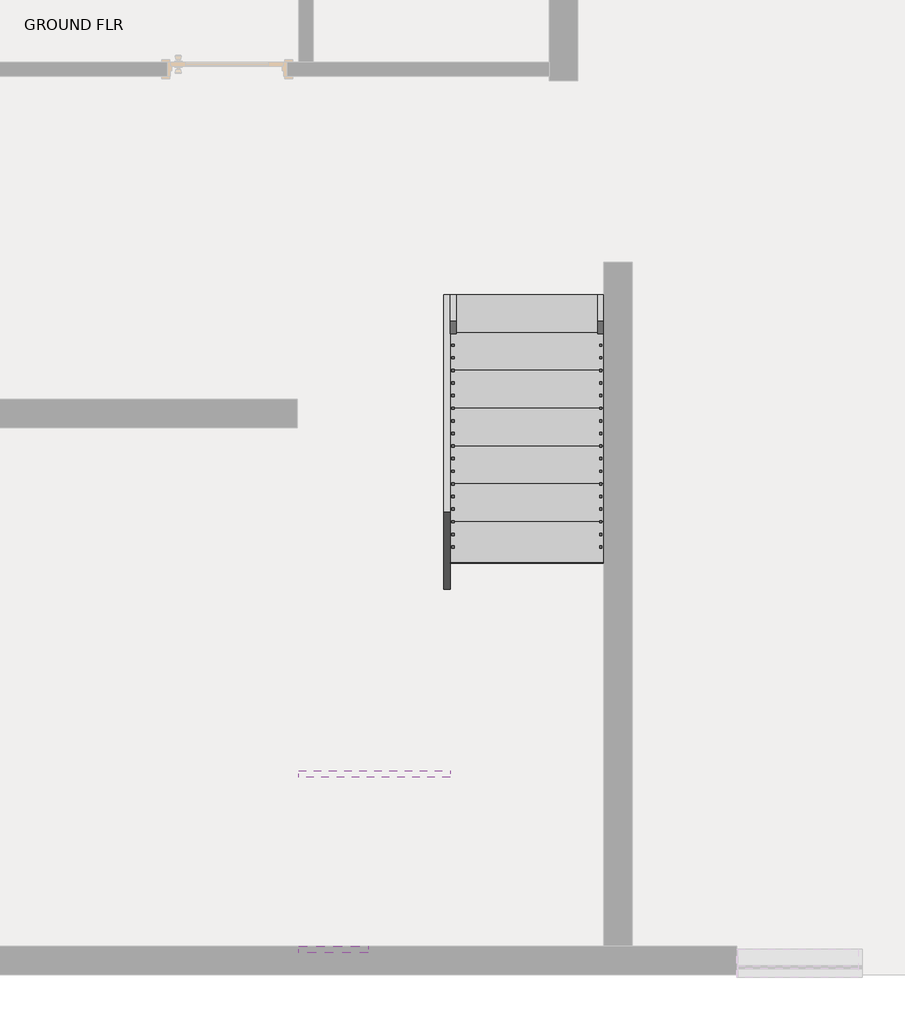
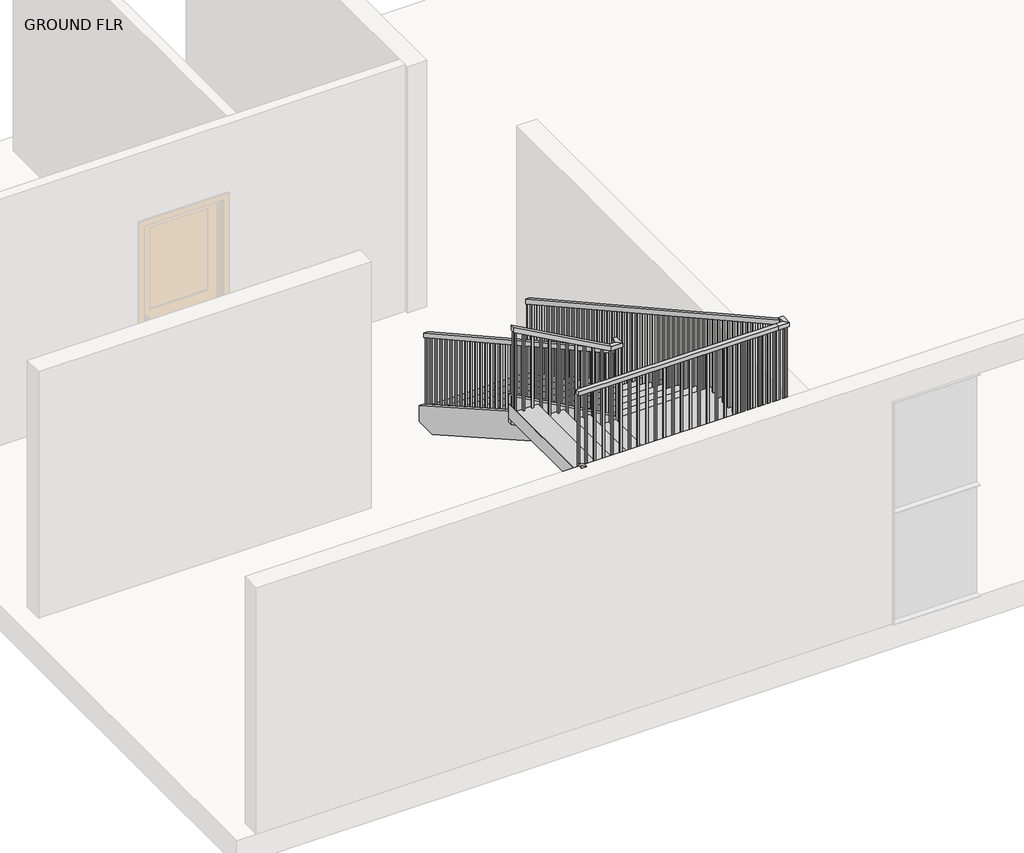
# One storey, part 3 of 3: 4 members, 2 railings, 1 stair flight.
"""IFC4 building model written with IfcOpenShell, lengths in millimetres."""

from ifc_helpers import new_model, si_unit, frame, origin, place, context, project, spatial, polyline, outline, extrude, faceted_brep, transform, mapped, element, save
from components import stair_flight_acf00c5d

model = new_model("IFC4")

# Units and contexts
model_context = context("Model", 3, world=origin())
ifc_project = project(units=[si_unit("LENGTHUNIT", "METRE", prefix="MILLI")], contexts=[model_context])

# Site, building, storey
site = spatial("IfcSite", under=ifc_project)
building = spatial("IfcBuilding", under=site)
storey = spatial("IfcBuildingStorey", under=building, Name="GROUND FLR", Elevation=304.8)

# Members
placement = place(None, origin())
element("IfcMember", 1, ObjectType="Stringer - 2\" Width", at=placement, inside=storey, context=model_context, shape_type="SweptSolid", body=[
    extrude(outline(polyline([(-746.7863315, 512.3983948), (-746.7863315, 304.8), (-1000.7308343, 304.8), (-4096.6287758, 2024.7433008), (-3469.0071624, 2024.7433008), (-746.7863315, 512.3983948)])), frame((-3766.7446058, 0.0, 0.0), z_axis=(1.0, 0.0, 0.0), x_axis=(0.0, 1.0, 0.0)), (0.0, 0.0, 1.0), 50.8),
])
element("IfcMember", 2, ObjectType="Stringer - 2\" Width", at=placement, inside=storey, context=model_context, shape_type="SweptSolid", body=[
    extrude(outline(polyline([(3080.0080444, -5666.2211442), (3391.0650614, -6226.1237749), (3080.0080444, -6226.1237749), (3080.0080444, -5666.2211442)])), frame((0.0, -6046.9053142, 0.0), z_axis=(0.0, 1.0, 0.0), x_axis=(0.0, 0.0, 1.0)), (0.0, 0.0, 1.0), 50.8),
])
element("IfcMember", 3, ObjectType="Stringer - 2\" Width", at=placement, inside=storey, context=model_context, shape_type="SweptSolid", body=[
    extrude(outline(polyline([(-746.7863315, 509.8166394), (-746.7863315, 304.8), (-1003.0994439, 304.8), (-4582.1863315, 2335.4875958), (-4582.1863315, 2685.9301146), (-746.7863315, 509.8166394)])), frame((-5057.7237749, 0.0, 0.0), z_axis=(1.0, 0.0, 0.0), x_axis=(0.0, 1.0, 0.0)), (0.0, 0.0, 1.0), 50.8),
])
element("IfcMember", 4, ObjectType="Stringer - 2\" Width", at=placement, inside=storey, context=model_context, shape_type="SweptSolid", body=[
    extrude(outline(polyline([(2365.053054, -5006.9237749), (2713.7317281, -5006.9237749), (3391.0650614, -6226.1237749), (3042.3863873, -6226.1237749), (2365.053054, -5006.9237749)])), frame((0.0, -4632.9863315, 0.0), z_axis=(0.0, 1.0, 0.0), x_axis=(0.0, 0.0, 1.0)), (0.0, 0.0, 1.0), 50.8),
])

# Railings
element("IfcRailing", 5, ObjectType="Handrail - Rectangular", at=placement, inside=storey, context=model_context, shape_type="SolidModel", body=[
    faceted_brep([(-4956.1237749, -746.7863315, 1388.5333333), (-4956.1237749, -746.7863315, 1330.420221), (-5006.9237749, -746.7863315, 1330.420221), (-5006.9237749, -746.7863315, 1388.5333333), (-4956.1237749, -4556.7863315, 3505.2), (-4956.1237749, -4607.5863315, 3475.3091099), (-5006.9237749, -4607.5863315, 3475.3091099), (-5006.9237749, -4556.7863315, 3505.2), (-4956.1237749, -4556.7863315, 3632.2), (-4956.1237749, -4607.5863315, 3581.4), (-5006.9237749, -4607.5863315, 3581.4), (-5006.9237749, -4556.7863315, 3632.2), (-4956.1237749, -4683.7863315, 3632.2), (-4956.1237749, -4683.7863315, 3581.4), (-5006.9237749, -4632.9863315, 3581.4), (-5006.9237749, -4632.9863315, 3632.2), (-5083.1237749, -4683.7863315, 3632.2), (-5096.2873772, -4683.7863315, 3581.4), (-5096.2873772, -4632.9863315, 3581.4), (-5083.1237749, -4632.9863315, 3632.2), (-6226.1237749, -4683.7863315, 4267.2), (-6226.1237749, -4632.9863315, 4267.2), (-6226.1237749, -4632.9863315, 4209.0868876), (-6226.1237749, -4683.7863315, 4209.0868876)], [[[0, 1, 2, 3]], [[1, 0, 4, 5]], [[2, 1, 5, 6]], [[3, 2, 6, 7]], [[0, 3, 7, 4]], [[5, 4, 8, 9]], [[6, 5, 9, 10]], [[7, 6, 10, 11]], [[4, 7, 11, 8]], [[9, 8, 12, 13]], [[10, 9, 13, 14]], [[11, 10, 14, 15]], [[8, 11, 15, 12]], [[13, 12, 16, 17]], [[14, 13, 17, 18]], [[15, 14, 18, 19]], [[12, 15, 19, 16]], [[20, 21, 22, 23]], [[17, 16, 20, 23]], [[18, 17, 23, 22]], [[19, 18, 22, 21]], [[16, 19, 21, 20]]]),
    extrude(outline(polyline([(4189.6841099, -6191.1987749), (4200.2674432, -6210.2487749), (3183.4666667, -6210.2487749), (3183.4666667, -6191.1987749), (4189.6841099, -6191.1987749)])), frame((0.0, -4667.9113315, 0.0), z_axis=(0.0, 1.0, 0.0), x_axis=(0.0, 0.0, 1.0)), (0.0, 0.0, 1.0), 19.05),
    extrude(outline(polyline([(4133.2396654, -6089.5987749), (4143.8229988, -6108.6487749), (3183.4666667, -6108.6487749), (3183.4666667, -6089.5987749), (4133.2396654, -6089.5987749)])), frame((0.0, -4667.9113315, 0.0), z_axis=(0.0, 1.0, 0.0), x_axis=(0.0, 0.0, 1.0)), (0.0, 0.0, 1.0), 19.05),
    extrude(outline(polyline([(4076.795221, -5987.9987749), (4087.3785543, -6007.0487749), (3183.4666667, -6007.0487749), (3183.4666667, -5987.9987749), (4076.795221, -5987.9987749)])), frame((0.0, -4667.9113315, 0.0), z_axis=(0.0, 1.0, 0.0), x_axis=(0.0, 0.0, 1.0)), (0.0, 0.0, 1.0), 19.05),
    extrude(outline(polyline([(4020.3507765, -5886.3987749), (4030.9341099, -5905.4487749), (3014.1333333, -5905.4487749), (3014.1333333, -5886.3987749), (4020.3507765, -5886.3987749)])), frame((0.0, -4667.9113315, 0.0), z_axis=(0.0, 1.0, 0.0), x_axis=(0.0, 0.0, 1.0)), (0.0, 0.0, 1.0), 19.05),
    extrude(outline(polyline([(3963.9063321, -5784.7987749), (3974.4896654, -5803.8487749), (3014.1333333, -5803.8487749), (3014.1333333, -5784.7987749), (3963.9063321, -5784.7987749)])), frame((0.0, -4667.9113315, 0.0), z_axis=(0.0, 1.0, 0.0), x_axis=(0.0, 0.0, 1.0)), (0.0, 0.0, 1.0), 19.05),
    extrude(outline(polyline([(3907.4618876, -5683.1987749), (3918.045221, -5702.2487749), (3014.1333333, -5702.2487749), (3014.1333333, -5683.1987749), (3907.4618876, -5683.1987749)])), frame((0.0, -4667.9113315, 0.0), z_axis=(0.0, 1.0, 0.0), x_axis=(0.0, 0.0, 1.0)), (0.0, 0.0, 1.0), 19.05),
    extrude(outline(polyline([(3851.0174432, -5581.5987749), (3861.6007765, -5600.6487749), (2844.8, -5600.6487749), (2844.8, -5581.5987749), (3851.0174432, -5581.5987749)])), frame((0.0, -4667.9113315, 0.0), z_axis=(0.0, 1.0, 0.0), x_axis=(0.0, 0.0, 1.0)), (0.0, 0.0, 1.0), 19.05),
    extrude(outline(polyline([(3794.5729988, -5479.9987749), (3805.1563321, -5499.0487749), (2844.8, -5499.0487749), (2844.8, -5479.9987749), (3794.5729988, -5479.9987749)])), frame((0.0, -4667.9113315, 0.0), z_axis=(0.0, 1.0, 0.0), x_axis=(0.0, 0.0, 1.0)), (0.0, 0.0, 1.0), 19.05),
    extrude(outline(polyline([(3738.1285543, -5378.3987749), (3748.7118876, -5397.4487749), (2844.8, -5397.4487749), (2844.8, -5378.3987749), (3738.1285543, -5378.3987749)])), frame((0.0, -4667.9113315, 0.0), z_axis=(0.0, 1.0, 0.0), x_axis=(0.0, 0.0, 1.0)), (0.0, 0.0, 1.0), 19.05),
    extrude(outline(polyline([(3681.6841099, -5276.7987749), (3692.2674432, -5295.8487749), (2675.4666667, -5295.8487749), (2675.4666667, -5276.7987749), (3681.6841099, -5276.7987749)])), frame((0.0, -4667.9113315, 0.0), z_axis=(0.0, 1.0, 0.0), x_axis=(0.0, 0.0, 1.0)), (0.0, 0.0, 1.0), 19.05),
    extrude(outline(polyline([(3625.2396654, -5175.1987749), (3635.8229988, -5194.2487749), (2675.4666667, -5194.2487749), (2675.4666667, -5175.1987749), (3625.2396654, -5175.1987749)])), frame((0.0, -4667.9113315, 0.0), z_axis=(0.0, 1.0, 0.0), x_axis=(0.0, 0.0, 1.0)), (0.0, 0.0, 1.0), 19.05),
    extrude(outline(polyline([(3568.795221, -5073.5987749), (3579.3785543, -5092.6487749), (2675.4666667, -5092.6487749), (2675.4666667, -5073.5987749), (3568.795221, -5073.5987749)])), frame((0.0, -4667.9113315, 0.0), z_axis=(0.0, 1.0, 0.0), x_axis=(0.0, 0.0, 1.0)), (0.0, 0.0, 1.0), 19.05),
    extrude(outline(polyline([(-4991.0487749, -4598.0613315), (-4971.9987749, -4598.0613315), (-4971.9987749, -4617.1113315), (-4991.0487749, -4617.1113315), (-4991.0487749, -4598.0613315)])), frame((0.0, 0.0, 2506.1333333), z_axis=(0.0, 0.0, 1.0), x_axis=(1.0, 0.0, 0.0)), (0.0, 0.0, 1.0), 1075.2666667),
    extrude(outline(polyline([(-4515.5113315, 3424.1563321), (-4496.4613315, 3413.5729988), (-4496.4613315, 2506.1333333), (-4515.5113315, 2506.1333333), (-4515.5113315, 3424.1563321)])), frame((-4991.0487749, 0.0, 0.0), z_axis=(1.0, 0.0, 0.0), x_axis=(0.0, 1.0, 0.0)), (0.0, 0.0, 1.0), 19.05),
    extrude(outline(polyline([(-4413.9113315, 3367.7118876), (-4394.8613315, 3357.1285543), (-4394.8613315, 2506.1333333), (-4413.9113315, 2506.1333333), (-4413.9113315, 3367.7118876)])), frame((-4991.0487749, 0.0, 0.0), z_axis=(1.0, 0.0, 0.0), x_axis=(0.0, 1.0, 0.0)), (0.0, 0.0, 1.0), 19.05),
    extrude(outline(polyline([(-4312.3113315, 3311.2674432), (-4293.2613315, 3300.6841099), (-4293.2613315, 2336.8), (-4312.3113315, 2336.8), (-4312.3113315, 3311.2674432)])), frame((-4991.0487749, 0.0, 0.0), z_axis=(1.0, 0.0, 0.0), x_axis=(0.0, 1.0, 0.0)), (0.0, 0.0, 1.0), 19.05),
    extrude(outline(polyline([(-4210.7113315, 3254.8229988), (-4191.6613315, 3244.2396654), (-4191.6613315, 2336.8), (-4210.7113315, 2336.8), (-4210.7113315, 3254.8229988)])), frame((-4991.0487749, 0.0, 0.0), z_axis=(1.0, 0.0, 0.0), x_axis=(0.0, 1.0, 0.0)), (0.0, 0.0, 1.0), 19.05),
    extrude(outline(polyline([(-4109.1113315, 3198.3785543), (-4090.0613315, 3187.795221), (-4090.0613315, 2336.8), (-4109.1113315, 2336.8), (-4109.1113315, 3198.3785543)])), frame((-4991.0487749, 0.0, 0.0), z_axis=(1.0, 0.0, 0.0), x_axis=(0.0, 1.0, 0.0)), (0.0, 0.0, 1.0), 19.05),
    extrude(outline(polyline([(-4007.5113315, 3141.9341099), (-3988.4613315, 3131.3507765), (-3988.4613315, 2167.4666667), (-4007.5113315, 2167.4666667), (-4007.5113315, 3141.9341099)])), frame((-4991.0487749, 0.0, 0.0), z_axis=(1.0, 0.0, 0.0), x_axis=(0.0, 1.0, 0.0)), (0.0, 0.0, 1.0), 19.05),
    extrude(outline(polyline([(-3905.9113315, 3085.4896654), (-3886.8613315, 3074.9063321), (-3886.8613315, 2167.4666667), (-3905.9113315, 2167.4666667), (-3905.9113315, 3085.4896654)])), frame((-4991.0487749, 0.0, 0.0), z_axis=(1.0, 0.0, 0.0), x_axis=(0.0, 1.0, 0.0)), (0.0, 0.0, 1.0), 19.05),
    extrude(outline(polyline([(-3804.3113315, 3029.045221), (-3785.2613315, 3018.4618876), (-3785.2613315, 2167.4666667), (-3804.3113315, 2167.4666667), (-3804.3113315, 3029.045221)])), frame((-4991.0487749, 0.0, 0.0), z_axis=(1.0, 0.0, 0.0), x_axis=(0.0, 1.0, 0.0)), (0.0, 0.0, 1.0), 19.05),
    extrude(outline(polyline([(-3702.7113315, 2972.6007765), (-3683.6613315, 2962.0174432), (-3683.6613315, 1998.1333333), (-3702.7113315, 1998.1333333), (-3702.7113315, 2972.6007765)])), frame((-4991.0487749, 0.0, 0.0), z_axis=(1.0, 0.0, 0.0), x_axis=(0.0, 1.0, 0.0)), (0.0, 0.0, 1.0), 19.05),
    extrude(outline(polyline([(-3601.1113315, 2916.1563321), (-3582.0613315, 2905.5729988), (-3582.0613315, 1998.1333333), (-3601.1113315, 1998.1333333), (-3601.1113315, 2916.1563321)])), frame((-4991.0487749, 0.0, 0.0), z_axis=(1.0, 0.0, 0.0), x_axis=(0.0, 1.0, 0.0)), (0.0, 0.0, 1.0), 19.05),
    extrude(outline(polyline([(-3499.5113315, 2859.7118876), (-3480.4613315, 2849.1285543), (-3480.4613315, 1998.1333333), (-3499.5113315, 1998.1333333), (-3499.5113315, 2859.7118876)])), frame((-4991.0487749, 0.0, 0.0), z_axis=(1.0, 0.0, 0.0), x_axis=(0.0, 1.0, 0.0)), (0.0, 0.0, 1.0), 19.05),
    extrude(outline(polyline([(-3397.9113315, 2803.2674432), (-3378.8613315, 2792.6841099), (-3378.8613315, 1828.8), (-3397.9113315, 1828.8), (-3397.9113315, 2803.2674432)])), frame((-4991.0487749, 0.0, 0.0), z_axis=(1.0, 0.0, 0.0), x_axis=(0.0, 1.0, 0.0)), (0.0, 0.0, 1.0), 19.05),
    extrude(outline(polyline([(-3296.3113315, 2746.8229988), (-3277.2613315, 2736.2396654), (-3277.2613315, 1828.8), (-3296.3113315, 1828.8), (-3296.3113315, 2746.8229988)])), frame((-4991.0487749, 0.0, 0.0), z_axis=(1.0, 0.0, 0.0), x_axis=(0.0, 1.0, 0.0)), (0.0, 0.0, 1.0), 19.05),
    extrude(outline(polyline([(-3194.7113315, 2690.3785543), (-3175.6613315, 2679.795221), (-3175.6613315, 1828.8), (-3194.7113315, 1828.8), (-3194.7113315, 2690.3785543)])), frame((-4991.0487749, 0.0, 0.0), z_axis=(1.0, 0.0, 0.0), x_axis=(0.0, 1.0, 0.0)), (0.0, 0.0, 1.0), 19.05),
    extrude(outline(polyline([(-3093.1113315, 2633.9341099), (-3074.0613315, 2623.3507765), (-3074.0613315, 1659.4666667), (-3093.1113315, 1659.4666667), (-3093.1113315, 2633.9341099)])), frame((-4991.0487749, 0.0, 0.0), z_axis=(1.0, 0.0, 0.0), x_axis=(0.0, 1.0, 0.0)), (0.0, 0.0, 1.0), 19.05),
    extrude(outline(polyline([(-2991.5113315, 2577.4896654), (-2972.4613315, 2566.9063321), (-2972.4613315, 1659.4666667), (-2991.5113315, 1659.4666667), (-2991.5113315, 2577.4896654)])), frame((-4991.0487749, 0.0, 0.0), z_axis=(1.0, 0.0, 0.0), x_axis=(0.0, 1.0, 0.0)), (0.0, 0.0, 1.0), 19.05),
    extrude(outline(polyline([(-2889.9113315, 2521.045221), (-2870.8613315, 2510.4618876), (-2870.8613315, 1659.4666667), (-2889.9113315, 1659.4666667), (-2889.9113315, 2521.045221)])), frame((-4991.0487749, 0.0, 0.0), z_axis=(1.0, 0.0, 0.0), x_axis=(0.0, 1.0, 0.0)), (0.0, 0.0, 1.0), 19.05),
    extrude(outline(polyline([(-2788.3113315, 2464.6007765), (-2769.2613315, 2454.0174432), (-2769.2613315, 1490.1333333), (-2788.3113315, 1490.1333333), (-2788.3113315, 2464.6007765)])), frame((-4991.0487749, 0.0, 0.0), z_axis=(1.0, 0.0, 0.0), x_axis=(0.0, 1.0, 0.0)), (0.0, 0.0, 1.0), 19.05),
    extrude(outline(polyline([(-2686.7113315, 2408.1563321), (-2667.6613315, 2397.5729988), (-2667.6613315, 1490.1333333), (-2686.7113315, 1490.1333333), (-2686.7113315, 2408.1563321)])), frame((-4991.0487749, 0.0, 0.0), z_axis=(1.0, 0.0, 0.0), x_axis=(0.0, 1.0, 0.0)), (0.0, 0.0, 1.0), 19.05),
    extrude(outline(polyline([(-2585.1113315, 2351.7118876), (-2566.0613315, 2341.1285543), (-2566.0613315, 1490.1333333), (-2585.1113315, 1490.1333333), (-2585.1113315, 2351.7118876)])), frame((-4991.0487749, 0.0, 0.0), z_axis=(1.0, 0.0, 0.0), x_axis=(0.0, 1.0, 0.0)), (0.0, 0.0, 1.0), 19.05),
    extrude(outline(polyline([(-2483.5113315, 2295.2674432), (-2464.4613315, 2284.6841099), (-2464.4613315, 1320.8), (-2483.5113315, 1320.8), (-2483.5113315, 2295.2674432)])), frame((-4991.0487749, 0.0, 0.0), z_axis=(1.0, 0.0, 0.0), x_axis=(0.0, 1.0, 0.0)), (0.0, 0.0, 1.0), 19.05),
    extrude(outline(polyline([(-2381.9113315, 2238.8229988), (-2362.8613315, 2228.2396654), (-2362.8613315, 1320.8), (-2381.9113315, 1320.8), (-2381.9113315, 2238.8229988)])), frame((-4991.0487749, 0.0, 0.0), z_axis=(1.0, 0.0, 0.0), x_axis=(0.0, 1.0, 0.0)), (0.0, 0.0, 1.0), 19.05),
    extrude(outline(polyline([(-2280.3113315, 2182.3785543), (-2261.2613315, 2171.795221), (-2261.2613315, 1320.8), (-2280.3113315, 1320.8), (-2280.3113315, 2182.3785543)])), frame((-4991.0487749, 0.0, 0.0), z_axis=(1.0, 0.0, 0.0), x_axis=(0.0, 1.0, 0.0)), (0.0, 0.0, 1.0), 19.05),
    extrude(outline(polyline([(-2178.7113315, 2125.9341099), (-2159.6613315, 2115.3507765), (-2159.6613315, 1151.4666667), (-2178.7113315, 1151.4666667), (-2178.7113315, 2125.9341099)])), frame((-4991.0487749, 0.0, 0.0), z_axis=(1.0, 0.0, 0.0), x_axis=(0.0, 1.0, 0.0)), (0.0, 0.0, 1.0), 19.05),
    extrude(outline(polyline([(-2077.1113315, 2069.4896654), (-2058.0613315, 2058.9063321), (-2058.0613315, 1151.4666667), (-2077.1113315, 1151.4666667), (-2077.1113315, 2069.4896654)])), frame((-4991.0487749, 0.0, 0.0), z_axis=(1.0, 0.0, 0.0), x_axis=(0.0, 1.0, 0.0)), (0.0, 0.0, 1.0), 19.05),
    extrude(outline(polyline([(-1975.5113315, 2013.045221), (-1956.4613315, 2002.4618876), (-1956.4613315, 1151.4666667), (-1975.5113315, 1151.4666667), (-1975.5113315, 2013.045221)])), frame((-4991.0487749, 0.0, 0.0), z_axis=(1.0, 0.0, 0.0), x_axis=(0.0, 1.0, 0.0)), (0.0, 0.0, 1.0), 19.05),
    extrude(outline(polyline([(-1873.9113315, 1956.6007765), (-1854.8613315, 1946.0174432), (-1854.8613315, 982.1333333), (-1873.9113315, 982.1333333), (-1873.9113315, 1956.6007765)])), frame((-4991.0487749, 0.0, 0.0), z_axis=(1.0, 0.0, 0.0), x_axis=(0.0, 1.0, 0.0)), (0.0, 0.0, 1.0), 19.05),
    extrude(outline(polyline([(-1772.3113315, 1900.1563321), (-1753.2613315, 1889.5729988), (-1753.2613315, 982.1333333), (-1772.3113315, 982.1333333), (-1772.3113315, 1900.1563321)])), frame((-4991.0487749, 0.0, 0.0), z_axis=(1.0, 0.0, 0.0), x_axis=(0.0, 1.0, 0.0)), (0.0, 0.0, 1.0), 19.05),
    extrude(outline(polyline([(-1670.7113315, 1843.7118876), (-1651.6613315, 1833.1285543), (-1651.6613315, 982.1333333), (-1670.7113315, 982.1333333), (-1670.7113315, 1843.7118876)])), frame((-4991.0487749, 0.0, 0.0), z_axis=(1.0, 0.0, 0.0), x_axis=(0.0, 1.0, 0.0)), (0.0, 0.0, 1.0), 19.05),
    extrude(outline(polyline([(-1569.1113315, 1787.2674432), (-1550.0613315, 1776.6841099), (-1550.0613315, 812.8), (-1569.1113315, 812.8), (-1569.1113315, 1787.2674432)])), frame((-4991.0487749, 0.0, 0.0), z_axis=(1.0, 0.0, 0.0), x_axis=(0.0, 1.0, 0.0)), (0.0, 0.0, 1.0), 19.05),
    extrude(outline(polyline([(-1467.5113315, 1730.8229988), (-1448.4613315, 1720.2396654), (-1448.4613315, 812.8), (-1467.5113315, 812.8), (-1467.5113315, 1730.8229988)])), frame((-4991.0487749, 0.0, 0.0), z_axis=(1.0, 0.0, 0.0), x_axis=(0.0, 1.0, 0.0)), (0.0, 0.0, 1.0), 19.05),
    extrude(outline(polyline([(-1365.9113315, 1674.3785543), (-1346.8613315, 1663.795221), (-1346.8613315, 812.8), (-1365.9113315, 812.8), (-1365.9113315, 1674.3785543)])), frame((-4991.0487749, 0.0, 0.0), z_axis=(1.0, 0.0, 0.0), x_axis=(0.0, 1.0, 0.0)), (0.0, 0.0, 1.0), 19.05),
    extrude(outline(polyline([(-1264.3113315, 1617.9341099), (-1245.2613315, 1607.3507765), (-1245.2613315, 643.4666667), (-1264.3113315, 643.4666667), (-1264.3113315, 1617.9341099)])), frame((-4991.0487749, 0.0, 0.0), z_axis=(1.0, 0.0, 0.0), x_axis=(0.0, 1.0, 0.0)), (0.0, 0.0, 1.0), 19.05),
    extrude(outline(polyline([(-1162.7113315, 1561.4896654), (-1143.6613315, 1550.9063321), (-1143.6613315, 643.4666667), (-1162.7113315, 643.4666667), (-1162.7113315, 1561.4896654)])), frame((-4991.0487749, 0.0, 0.0), z_axis=(1.0, 0.0, 0.0), x_axis=(0.0, 1.0, 0.0)), (0.0, 0.0, 1.0), 19.05),
    extrude(outline(polyline([(-1061.1113315, 1505.045221), (-1042.0613315, 1494.4618876), (-1042.0613315, 643.4666667), (-1061.1113315, 643.4666667), (-1061.1113315, 1505.045221)])), frame((-4991.0487749, 0.0, 0.0), z_axis=(1.0, 0.0, 0.0), x_axis=(0.0, 1.0, 0.0)), (0.0, 0.0, 1.0), 19.05),
    extrude(outline(polyline([(-959.5113315, 1448.6007765), (-940.4613315, 1438.0174432), (-940.4613315, 474.1333333), (-959.5113315, 474.1333333), (-959.5113315, 1448.6007765)])), frame((-4991.0487749, 0.0, 0.0), z_axis=(1.0, 0.0, 0.0), x_axis=(0.0, 1.0, 0.0)), (0.0, 0.0, 1.0), 19.05),
    extrude(outline(polyline([(-857.9113315, 1392.1563321), (-838.8613315, 1381.5729988), (-838.8613315, 474.1333333), (-857.9113315, 474.1333333), (-857.9113315, 1392.1563321)])), frame((-4991.0487749, 0.0, 0.0), z_axis=(1.0, 0.0, 0.0), x_axis=(0.0, 1.0, 0.0)), (0.0, 0.0, 1.0), 19.05),
    extrude(outline(polyline([(-4991.0487749, -4648.8613315), (-4971.9987749, -4648.8613315), (-4971.9987749, -4667.9113315), (-4991.0487749, -4667.9113315), (-4991.0487749, -4648.8613315)])), frame((0.0, 0.0, 2506.1333333), z_axis=(0.0, 0.0, 1.0), x_axis=(1.0, 0.0, 0.0)), (0.0, 0.0, 1.0), 1075.2666667),
    extrude(outline(polyline([(4198.5035543, -6207.0737749), (4209.0868876, -6226.1237749), (3183.4666667, -6226.1237749), (3183.4666667, -6207.0737749), (4198.5035543, -6207.0737749)])), frame((0.0, -4667.9113315, 0.0), z_axis=(0.0, 1.0, 0.0), x_axis=(0.0, 0.0, 1.0)), (0.0, 0.0, 1.0), 19.05),
    extrude(outline(polyline([(-765.8363315, 1341.0035543), (-746.7863315, 1330.420221), (-746.7863315, 474.1333333), (-765.8363315, 474.1333333), (-765.8363315, 1341.0035543)])), frame((-4991.0487749, 0.0, 0.0), z_axis=(1.0, 0.0, 0.0), x_axis=(0.0, 1.0, 0.0)), (0.0, 0.0, 1.0), 19.05),
])
element("IfcRailing", 6, ObjectType="Handrail - Rectangular", at=placement, inside=storey, context=model_context, shape_type="SolidModel", body=[
    faceted_brep([(-3766.7446058, -746.7863315, 1388.5333333), (-3766.7446058, -746.7863315, 1330.420221), (-3817.5446058, -746.7863315, 1330.420221), (-3817.5446058, -746.7863315, 1388.5333333), (-3766.7446058, -5869.1053142, 4234.2661015), (-3766.7446058, -5919.9053142, 4204.3752114), (-3817.5446058, -5919.9053142, 4204.3752114), (-3817.5446058, -5869.1053142, 4234.2661015), (-3766.7446058, -5869.1053142, 4267.2), (-3766.7446058, -5919.9053142, 4216.4), (-3817.5446058, -5919.9053142, 4216.4), (-3817.5446058, -5869.1053142, 4267.2), (-3766.7446058, -5996.1053142, 4267.2), (-3766.7446058, -5996.1053142, 4216.4), (-3817.5446058, -5945.3053142, 4216.4), (-3817.5446058, -5945.3053142, 4267.2), (-3893.7446058, -5996.1053142, 4267.2), (-3893.7446058, -5996.1053142, 4216.4), (-3893.7446058, -5945.3053142, 4216.4), (-3893.7446058, -5945.3053142, 4267.2), (-6226.1237749, -5996.1053142, 4267.2), (-6226.1237749, -5945.3053142, 4267.2), (-6226.1237749, -5945.3053142, 4216.4), (-6226.1237749, -5996.1053142, 4216.4)], [[[0, 1, 2, 3]], [[1, 0, 4, 5]], [[2, 1, 5, 6]], [[3, 2, 6, 7]], [[0, 3, 7, 4]], [[5, 4, 8, 9]], [[6, 5, 9, 10]], [[7, 6, 10, 11]], [[4, 7, 11, 8]], [[9, 8, 12, 13]], [[10, 9, 13, 14]], [[11, 10, 14, 15]], [[8, 11, 15, 12]], [[13, 12, 16, 17]], [[14, 13, 17, 18]], [[15, 14, 18, 19]], [[12, 15, 19, 16]], [[20, 21, 22, 23]], [[17, 16, 20, 23]], [[18, 17, 23, 22]], [[19, 18, 22, 21]], [[16, 19, 21, 20]]]),
    extrude(outline(polyline([(-6119.4196058, -5980.2303142), (-6138.4696058, -5980.2303142), (-6138.4696058, -5961.1803142), (-6119.4196058, -5961.1803142), (-6119.4196058, -5980.2303142)])), frame((0.0, 0.0, 3183.4666667), z_axis=(0.0, 0.0, 1.0), x_axis=(1.0, 0.0, 0.0)), (0.0, 0.0, 1.0), 1032.9333333),
    extrude(outline(polyline([(-6017.8196058, -5980.2303142), (-6036.8696058, -5980.2303142), (-6036.8696058, -5961.1803142), (-6017.8196058, -5961.1803142), (-6017.8196058, -5980.2303142)])), frame((0.0, 0.0, 3183.4666667), z_axis=(0.0, 0.0, 1.0), x_axis=(1.0, 0.0, 0.0)), (0.0, 0.0, 1.0), 1032.9333333),
    extrude(outline(polyline([(-5916.2196058, -5980.2303142), (-5935.2696058, -5980.2303142), (-5935.2696058, -5961.1803142), (-5916.2196058, -5961.1803142), (-5916.2196058, -5980.2303142)])), frame((0.0, 0.0, 3183.4666667), z_axis=(0.0, 0.0, 1.0), x_axis=(1.0, 0.0, 0.0)), (0.0, 0.0, 1.0), 1032.9333333),
    extrude(outline(polyline([(-5814.6196058, -5980.2303142), (-5833.6696058, -5980.2303142), (-5833.6696058, -5961.1803142), (-5814.6196058, -5961.1803142), (-5814.6196058, -5980.2303142)])), frame((0.0, 0.0, 3014.1333333), z_axis=(0.0, 0.0, 1.0), x_axis=(1.0, 0.0, 0.0)), (0.0, 0.0, 1.0), 1202.2666667),
    extrude(outline(polyline([(-5713.0196058, -5980.2303142), (-5732.0696058, -5980.2303142), (-5732.0696058, -5961.1803142), (-5713.0196058, -5961.1803142), (-5713.0196058, -5980.2303142)])), frame((0.0, 0.0, 3014.1333333), z_axis=(0.0, 0.0, 1.0), x_axis=(1.0, 0.0, 0.0)), (0.0, 0.0, 1.0), 1202.2666667),
    extrude(outline(polyline([(-5611.4196058, -5980.2303142), (-5630.4696058, -5980.2303142), (-5630.4696058, -5961.1803142), (-5611.4196058, -5961.1803142), (-5611.4196058, -5980.2303142)])), frame((0.0, 0.0, 3014.1333333), z_axis=(0.0, 0.0, 1.0), x_axis=(1.0, 0.0, 0.0)), (0.0, 0.0, 1.0), 1202.2666667),
    extrude(outline(polyline([(-5509.8196058, -5980.2303142), (-5528.8696058, -5980.2303142), (-5528.8696058, -5961.1803142), (-5509.8196058, -5961.1803142), (-5509.8196058, -5980.2303142)])), frame((0.0, 0.0, 2844.8), z_axis=(0.0, 0.0, 1.0), x_axis=(1.0, 0.0, 0.0)), (0.0, 0.0, 1.0), 1371.6),
    extrude(outline(polyline([(-5408.2196058, -5980.2303142), (-5427.2696058, -5980.2303142), (-5427.2696058, -5961.1803142), (-5408.2196058, -5961.1803142), (-5408.2196058, -5980.2303142)])), frame((0.0, 0.0, 2844.8), z_axis=(0.0, 0.0, 1.0), x_axis=(1.0, 0.0, 0.0)), (0.0, 0.0, 1.0), 1371.6),
    extrude(outline(polyline([(-5306.6196058, -5980.2303142), (-5325.6696058, -5980.2303142), (-5325.6696058, -5961.1803142), (-5306.6196058, -5961.1803142), (-5306.6196058, -5980.2303142)])), frame((0.0, 0.0, 2844.8), z_axis=(0.0, 0.0, 1.0), x_axis=(1.0, 0.0, 0.0)), (0.0, 0.0, 1.0), 1371.6),
    extrude(outline(polyline([(-5205.0196058, -5980.2303142), (-5224.0696058, -5980.2303142), (-5224.0696058, -5961.1803142), (-5205.0196058, -5961.1803142), (-5205.0196058, -5980.2303142)])), frame((0.0, 0.0, 2675.4666667), z_axis=(0.0, 0.0, 1.0), x_axis=(1.0, 0.0, 0.0)), (0.0, 0.0, 1.0), 1540.9333333),
    extrude(outline(polyline([(-5103.4196058, -5980.2303142), (-5122.4696058, -5980.2303142), (-5122.4696058, -5961.1803142), (-5103.4196058, -5961.1803142), (-5103.4196058, -5980.2303142)])), frame((0.0, 0.0, 2675.4666667), z_axis=(0.0, 0.0, 1.0), x_axis=(1.0, 0.0, 0.0)), (0.0, 0.0, 1.0), 1540.9333333),
    extrude(outline(polyline([(-5001.8196058, -5980.2303142), (-5020.8696058, -5980.2303142), (-5020.8696058, -5961.1803142), (-5001.8196058, -5961.1803142), (-5001.8196058, -5980.2303142)])), frame((0.0, 0.0, 2675.4666667), z_axis=(0.0, 0.0, 1.0), x_axis=(1.0, 0.0, 0.0)), (0.0, 0.0, 1.0), 1540.9333333),
    extrude(outline(polyline([(-4900.2196058, -5980.2303142), (-4919.2696058, -5980.2303142), (-4919.2696058, -5961.1803142), (-4900.2196058, -5961.1803142), (-4900.2196058, -5980.2303142)])), frame((0.0, 0.0, 2506.1333333), z_axis=(0.0, 0.0, 1.0), x_axis=(1.0, 0.0, 0.0)), (0.0, 0.0, 1.0), 1710.2666667),
    extrude(outline(polyline([(-4798.6196058, -5980.2303142), (-4817.6696058, -5980.2303142), (-4817.6696058, -5961.1803142), (-4798.6196058, -5961.1803142), (-4798.6196058, -5980.2303142)])), frame((0.0, 0.0, 2506.1333333), z_axis=(0.0, 0.0, 1.0), x_axis=(1.0, 0.0, 0.0)), (0.0, 0.0, 1.0), 1710.2666667),
    extrude(outline(polyline([(-4697.0196058, -5980.2303142), (-4716.0696058, -5980.2303142), (-4716.0696058, -5961.1803142), (-4697.0196058, -5961.1803142), (-4697.0196058, -5980.2303142)])), frame((0.0, 0.0, 2506.1333333), z_axis=(0.0, 0.0, 1.0), x_axis=(1.0, 0.0, 0.0)), (0.0, 0.0, 1.0), 1710.2666667),
    extrude(outline(polyline([(-4595.4196058, -5980.2303142), (-4614.4696058, -5980.2303142), (-4614.4696058, -5961.1803142), (-4595.4196058, -5961.1803142), (-4595.4196058, -5980.2303142)])), frame((0.0, 0.0, 2506.1333333), z_axis=(0.0, 0.0, 1.0), x_axis=(1.0, 0.0, 0.0)), (0.0, 0.0, 1.0), 1710.2666667),
    extrude(outline(polyline([(-4493.8196058, -5980.2303142), (-4512.8696058, -5980.2303142), (-4512.8696058, -5961.1803142), (-4493.8196058, -5961.1803142), (-4493.8196058, -5980.2303142)])), frame((0.0, 0.0, 2506.1333333), z_axis=(0.0, 0.0, 1.0), x_axis=(1.0, 0.0, 0.0)), (0.0, 0.0, 1.0), 1710.2666667),
    extrude(outline(polyline([(-4392.2196058, -5980.2303142), (-4411.2696058, -5980.2303142), (-4411.2696058, -5961.1803142), (-4392.2196058, -5961.1803142), (-4392.2196058, -5980.2303142)])), frame((0.0, 0.0, 2506.1333333), z_axis=(0.0, 0.0, 1.0), x_axis=(1.0, 0.0, 0.0)), (0.0, 0.0, 1.0), 1710.2666667),
    extrude(outline(polyline([(-4290.6196058, -5980.2303142), (-4309.6696058, -5980.2303142), (-4309.6696058, -5961.1803142), (-4290.6196058, -5961.1803142), (-4290.6196058, -5980.2303142)])), frame((0.0, 0.0, 2506.1333333), z_axis=(0.0, 0.0, 1.0), x_axis=(1.0, 0.0, 0.0)), (0.0, 0.0, 1.0), 1710.2666667),
    extrude(outline(polyline([(-4189.0196058, -5980.2303142), (-4208.0696058, -5980.2303142), (-4208.0696058, -5961.1803142), (-4189.0196058, -5961.1803142), (-4189.0196058, -5980.2303142)])), frame((0.0, 0.0, 2506.1333333), z_axis=(0.0, 0.0, 1.0), x_axis=(1.0, 0.0, 0.0)), (0.0, 0.0, 1.0), 1710.2666667),
    extrude(outline(polyline([(-4087.4196058, -5980.2303142), (-4106.4696058, -5980.2303142), (-4106.4696058, -5961.1803142), (-4087.4196058, -5961.1803142), (-4087.4196058, -5980.2303142)])), frame((0.0, 0.0, 2506.1333333), z_axis=(0.0, 0.0, 1.0), x_axis=(1.0, 0.0, 0.0)), (0.0, 0.0, 1.0), 1710.2666667),
    extrude(outline(polyline([(-3985.8196058, -5980.2303142), (-4004.8696058, -5980.2303142), (-4004.8696058, -5961.1803142), (-3985.8196058, -5961.1803142), (-3985.8196058, -5980.2303142)])), frame((0.0, 0.0, 2506.1333333), z_axis=(0.0, 0.0, 1.0), x_axis=(1.0, 0.0, 0.0)), (0.0, 0.0, 1.0), 1710.2666667),
    extrude(outline(polyline([(-3884.2196058, -5980.2303142), (-3903.2696058, -5980.2303142), (-3903.2696058, -5961.1803142), (-3884.2196058, -5961.1803142), (-3884.2196058, -5980.2303142)])), frame((0.0, 0.0, 2506.1333333), z_axis=(0.0, 0.0, 1.0), x_axis=(1.0, 0.0, 0.0)), (0.0, 0.0, 1.0), 1710.2666667),
    extrude(outline(polyline([(-3782.6196058, -5918.8613315), (-3782.6196058, -5937.9113315), (-3801.6696058, -5937.9113315), (-3801.6696058, -5918.8613315), (-3782.6196058, -5918.8613315)])), frame((0.0, 0.0, 2506.1333333), z_axis=(0.0, 0.0, 1.0), x_axis=(1.0, 0.0, 0.0)), (0.0, 0.0, 1.0), 1710.2666667),
    extrude(outline(polyline([(-5817.2613315, 4147.3507765), (-5817.2613315, 2506.1333333), (-5836.3113315, 2506.1333333), (-5836.3113315, 4157.9341099), (-5817.2613315, 4147.3507765)])), frame((-3801.6696058, 0.0, 0.0), z_axis=(1.0, 0.0, 0.0), x_axis=(0.0, 1.0, 0.0)), (0.0, 0.0, 1.0), 19.05),
    extrude(outline(polyline([(-5715.6613315, 4090.9063321), (-5715.6613315, 2506.1333333), (-5734.7113315, 2506.1333333), (-5734.7113315, 4101.4896654), (-5715.6613315, 4090.9063321)])), frame((-3801.6696058, 0.0, 0.0), z_axis=(1.0, 0.0, 0.0), x_axis=(0.0, 1.0, 0.0)), (0.0, 0.0, 1.0), 19.05),
    extrude(outline(polyline([(-5614.0613315, 4034.4618876), (-5614.0613315, 2506.1333333), (-5633.1113315, 2506.1333333), (-5633.1113315, 4045.045221), (-5614.0613315, 4034.4618876)])), frame((-3801.6696058, 0.0, 0.0), z_axis=(1.0, 0.0, 0.0), x_axis=(0.0, 1.0, 0.0)), (0.0, 0.0, 1.0), 19.05),
    extrude(outline(polyline([(-5512.4613315, 3978.0174432), (-5512.4613315, 2506.1333333), (-5531.5113315, 2506.1333333), (-5531.5113315, 3988.6007765), (-5512.4613315, 3978.0174432)])), frame((-3801.6696058, 0.0, 0.0), z_axis=(1.0, 0.0, 0.0), x_axis=(0.0, 1.0, 0.0)), (0.0, 0.0, 1.0), 19.05),
    extrude(outline(polyline([(-5410.8613315, 3921.5729988), (-5410.8613315, 2506.1333333), (-5429.9113315, 2506.1333333), (-5429.9113315, 3932.1563321), (-5410.8613315, 3921.5729988)])), frame((-3801.6696058, 0.0, 0.0), z_axis=(1.0, 0.0, 0.0), x_axis=(0.0, 1.0, 0.0)), (0.0, 0.0, 1.0), 19.05),
    extrude(outline(polyline([(-5309.2613315, 3865.1285543), (-5309.2613315, 2506.1333333), (-5328.3113315, 2506.1333333), (-5328.3113315, 3875.7118876), (-5309.2613315, 3865.1285543)])), frame((-3801.6696058, 0.0, 0.0), z_axis=(1.0, 0.0, 0.0), x_axis=(0.0, 1.0, 0.0)), (0.0, 0.0, 1.0), 19.05),
    extrude(outline(polyline([(-5207.6613315, 3808.6841099), (-5207.6613315, 2506.1333333), (-5226.7113315, 2506.1333333), (-5226.7113315, 3819.2674432), (-5207.6613315, 3808.6841099)])), frame((-3801.6696058, 0.0, 0.0), z_axis=(1.0, 0.0, 0.0), x_axis=(0.0, 1.0, 0.0)), (0.0, 0.0, 1.0), 19.05),
    extrude(outline(polyline([(-5106.0613315, 3752.2396654), (-5106.0613315, 2506.1333333), (-5125.1113315, 2506.1333333), (-5125.1113315, 3762.8229988), (-5106.0613315, 3752.2396654)])), frame((-3801.6696058, 0.0, 0.0), z_axis=(1.0, 0.0, 0.0), x_axis=(0.0, 1.0, 0.0)), (0.0, 0.0, 1.0), 19.05),
    extrude(outline(polyline([(-5004.4613315, 3695.795221), (-5004.4613315, 2506.1333333), (-5023.5113315, 2506.1333333), (-5023.5113315, 3706.3785543), (-5004.4613315, 3695.795221)])), frame((-3801.6696058, 0.0, 0.0), z_axis=(1.0, 0.0, 0.0), x_axis=(0.0, 1.0, 0.0)), (0.0, 0.0, 1.0), 19.05),
    extrude(outline(polyline([(-4902.8613315, 3639.3507765), (-4902.8613315, 2506.1333333), (-4921.9113315, 2506.1333333), (-4921.9113315, 3649.9341099), (-4902.8613315, 3639.3507765)])), frame((-3801.6696058, 0.0, 0.0), z_axis=(1.0, 0.0, 0.0), x_axis=(0.0, 1.0, 0.0)), (0.0, 0.0, 1.0), 19.05),
    extrude(outline(polyline([(-4801.2613315, 3582.9063321), (-4801.2613315, 2506.1333333), (-4820.3113315, 2506.1333333), (-4820.3113315, 3593.4896654), (-4801.2613315, 3582.9063321)])), frame((-3801.6696058, 0.0, 0.0), z_axis=(1.0, 0.0, 0.0), x_axis=(0.0, 1.0, 0.0)), (0.0, 0.0, 1.0), 19.05),
    extrude(outline(polyline([(-4699.6613315, 3526.4618876), (-4699.6613315, 2506.1333333), (-4718.7113315, 2506.1333333), (-4718.7113315, 3537.045221), (-4699.6613315, 3526.4618876)])), frame((-3801.6696058, 0.0, 0.0), z_axis=(1.0, 0.0, 0.0), x_axis=(0.0, 1.0, 0.0)), (0.0, 0.0, 1.0), 19.05),
    extrude(outline(polyline([(-4598.0613315, 3470.0174432), (-4598.0613315, 2506.1333333), (-4617.1113315, 2506.1333333), (-4617.1113315, 3480.6007765), (-4598.0613315, 3470.0174432)])), frame((-3801.6696058, 0.0, 0.0), z_axis=(1.0, 0.0, 0.0), x_axis=(0.0, 1.0, 0.0)), (0.0, 0.0, 1.0), 19.05),
    extrude(outline(polyline([(-4496.4613315, 3413.5729988), (-4496.4613315, 2506.1333333), (-4515.5113315, 2506.1333333), (-4515.5113315, 3424.1563321), (-4496.4613315, 3413.5729988)])), frame((-3801.6696058, 0.0, 0.0), z_axis=(1.0, 0.0, 0.0), x_axis=(0.0, 1.0, 0.0)), (0.0, 0.0, 1.0), 19.05),
    extrude(outline(polyline([(-4394.8613315, 3357.1285543), (-4394.8613315, 2506.1333333), (-4413.9113315, 2506.1333333), (-4413.9113315, 3367.7118876), (-4394.8613315, 3357.1285543)])), frame((-3801.6696058, 0.0, 0.0), z_axis=(1.0, 0.0, 0.0), x_axis=(0.0, 1.0, 0.0)), (0.0, 0.0, 1.0), 19.05),
    extrude(outline(polyline([(-4293.2613315, 3300.6841099), (-4293.2613315, 2336.8), (-4312.3113315, 2336.8), (-4312.3113315, 3311.2674432), (-4293.2613315, 3300.6841099)])), frame((-3801.6696058, 0.0, 0.0), z_axis=(1.0, 0.0, 0.0), x_axis=(0.0, 1.0, 0.0)), (0.0, 0.0, 1.0), 19.05),
    extrude(outline(polyline([(-4191.6613315, 3244.2396654), (-4191.6613315, 2336.8), (-4210.7113315, 2336.8), (-4210.7113315, 3254.8229988), (-4191.6613315, 3244.2396654)])), frame((-3801.6696058, 0.0, 0.0), z_axis=(1.0, 0.0, 0.0), x_axis=(0.0, 1.0, 0.0)), (0.0, 0.0, 1.0), 19.05),
    extrude(outline(polyline([(-4090.0613315, 3187.795221), (-4090.0613315, 2336.8), (-4109.1113315, 2336.8), (-4109.1113315, 3198.3785543), (-4090.0613315, 3187.795221)])), frame((-3801.6696058, 0.0, 0.0), z_axis=(1.0, 0.0, 0.0), x_axis=(0.0, 1.0, 0.0)), (0.0, 0.0, 1.0), 19.05),
    extrude(outline(polyline([(-3988.4613315, 3131.3507765), (-3988.4613315, 2167.4666667), (-4007.5113315, 2167.4666667), (-4007.5113315, 3141.9341099), (-3988.4613315, 3131.3507765)])), frame((-3801.6696058, 0.0, 0.0), z_axis=(1.0, 0.0, 0.0), x_axis=(0.0, 1.0, 0.0)), (0.0, 0.0, 1.0), 19.05),
    extrude(outline(polyline([(-3886.8613315, 3074.9063321), (-3886.8613315, 2167.4666667), (-3905.9113315, 2167.4666667), (-3905.9113315, 3085.4896654), (-3886.8613315, 3074.9063321)])), frame((-3801.6696058, 0.0, 0.0), z_axis=(1.0, 0.0, 0.0), x_axis=(0.0, 1.0, 0.0)), (0.0, 0.0, 1.0), 19.05),
    extrude(outline(polyline([(-3785.2613315, 3018.4618876), (-3785.2613315, 2167.4666667), (-3804.3113315, 2167.4666667), (-3804.3113315, 3029.045221), (-3785.2613315, 3018.4618876)])), frame((-3801.6696058, 0.0, 0.0), z_axis=(1.0, 0.0, 0.0), x_axis=(0.0, 1.0, 0.0)), (0.0, 0.0, 1.0), 19.05),
    extrude(outline(polyline([(-3683.6613315, 2962.0174432), (-3683.6613315, 1998.1333333), (-3702.7113315, 1998.1333333), (-3702.7113315, 2972.6007765), (-3683.6613315, 2962.0174432)])), frame((-3801.6696058, 0.0, 0.0), z_axis=(1.0, 0.0, 0.0), x_axis=(0.0, 1.0, 0.0)), (0.0, 0.0, 1.0), 19.05),
    extrude(outline(polyline([(-3582.0613315, 2905.5729988), (-3582.0613315, 1998.1333333), (-3601.1113315, 1998.1333333), (-3601.1113315, 2916.1563321), (-3582.0613315, 2905.5729988)])), frame((-3801.6696058, 0.0, 0.0), z_axis=(1.0, 0.0, 0.0), x_axis=(0.0, 1.0, 0.0)), (0.0, 0.0, 1.0), 19.05),
    extrude(outline(polyline([(-3480.4613315, 2849.1285543), (-3480.4613315, 1998.1333333), (-3499.5113315, 1998.1333333), (-3499.5113315, 2859.7118876), (-3480.4613315, 2849.1285543)])), frame((-3801.6696058, 0.0, 0.0), z_axis=(1.0, 0.0, 0.0), x_axis=(0.0, 1.0, 0.0)), (0.0, 0.0, 1.0), 19.05),
    extrude(outline(polyline([(-3378.8613315, 2792.6841099), (-3378.8613315, 1828.8), (-3397.9113315, 1828.8), (-3397.9113315, 2803.2674432), (-3378.8613315, 2792.6841099)])), frame((-3801.6696058, 0.0, 0.0), z_axis=(1.0, 0.0, 0.0), x_axis=(0.0, 1.0, 0.0)), (0.0, 0.0, 1.0), 19.05),
    extrude(outline(polyline([(-3277.2613315, 2736.2396654), (-3277.2613315, 1828.8), (-3296.3113315, 1828.8), (-3296.3113315, 2746.8229988), (-3277.2613315, 2736.2396654)])), frame((-3801.6696058, 0.0, 0.0), z_axis=(1.0, 0.0, 0.0), x_axis=(0.0, 1.0, 0.0)), (0.0, 0.0, 1.0), 19.05),
    extrude(outline(polyline([(-3175.6613315, 2679.795221), (-3175.6613315, 1828.8), (-3194.7113315, 1828.8), (-3194.7113315, 2690.3785543), (-3175.6613315, 2679.795221)])), frame((-3801.6696058, 0.0, 0.0), z_axis=(1.0, 0.0, 0.0), x_axis=(0.0, 1.0, 0.0)), (0.0, 0.0, 1.0), 19.05),
    extrude(outline(polyline([(-3074.0613315, 2623.3507765), (-3074.0613315, 1659.4666667), (-3093.1113315, 1659.4666667), (-3093.1113315, 2633.9341099), (-3074.0613315, 2623.3507765)])), frame((-3801.6696058, 0.0, 0.0), z_axis=(1.0, 0.0, 0.0), x_axis=(0.0, 1.0, 0.0)), (0.0, 0.0, 1.0), 19.05),
    extrude(outline(polyline([(-2972.4613315, 2566.9063321), (-2972.4613315, 1659.4666667), (-2991.5113315, 1659.4666667), (-2991.5113315, 2577.4896654), (-2972.4613315, 2566.9063321)])), frame((-3801.6696058, 0.0, 0.0), z_axis=(1.0, 0.0, 0.0), x_axis=(0.0, 1.0, 0.0)), (0.0, 0.0, 1.0), 19.05),
    extrude(outline(polyline([(-2870.8613315, 2510.4618876), (-2870.8613315, 1659.4666667), (-2889.9113315, 1659.4666667), (-2889.9113315, 2521.045221), (-2870.8613315, 2510.4618876)])), frame((-3801.6696058, 0.0, 0.0), z_axis=(1.0, 0.0, 0.0), x_axis=(0.0, 1.0, 0.0)), (0.0, 0.0, 1.0), 19.05),
    extrude(outline(polyline([(-2769.2613315, 2454.0174432), (-2769.2613315, 1490.1333333), (-2788.3113315, 1490.1333333), (-2788.3113315, 2464.6007765), (-2769.2613315, 2454.0174432)])), frame((-3801.6696058, 0.0, 0.0), z_axis=(1.0, 0.0, 0.0), x_axis=(0.0, 1.0, 0.0)), (0.0, 0.0, 1.0), 19.05),
    extrude(outline(polyline([(-2667.6613315, 2397.5729988), (-2667.6613315, 1490.1333333), (-2686.7113315, 1490.1333333), (-2686.7113315, 2408.1563321), (-2667.6613315, 2397.5729988)])), frame((-3801.6696058, 0.0, 0.0), z_axis=(1.0, 0.0, 0.0), x_axis=(0.0, 1.0, 0.0)), (0.0, 0.0, 1.0), 19.05),
    extrude(outline(polyline([(-2566.0613315, 2341.1285543), (-2566.0613315, 1490.1333333), (-2585.1113315, 1490.1333333), (-2585.1113315, 2351.7118876), (-2566.0613315, 2341.1285543)])), frame((-3801.6696058, 0.0, 0.0), z_axis=(1.0, 0.0, 0.0), x_axis=(0.0, 1.0, 0.0)), (0.0, 0.0, 1.0), 19.05),
    extrude(outline(polyline([(-2464.4613315, 2284.6841099), (-2464.4613315, 1320.8), (-2483.5113315, 1320.8), (-2483.5113315, 2295.2674432), (-2464.4613315, 2284.6841099)])), frame((-3801.6696058, 0.0, 0.0), z_axis=(1.0, 0.0, 0.0), x_axis=(0.0, 1.0, 0.0)), (0.0, 0.0, 1.0), 19.05),
    extrude(outline(polyline([(-2362.8613315, 2228.2396654), (-2362.8613315, 1320.8), (-2381.9113315, 1320.8), (-2381.9113315, 2238.8229988), (-2362.8613315, 2228.2396654)])), frame((-3801.6696058, 0.0, 0.0), z_axis=(1.0, 0.0, 0.0), x_axis=(0.0, 1.0, 0.0)), (0.0, 0.0, 1.0), 19.05),
    extrude(outline(polyline([(-2261.2613315, 2171.795221), (-2261.2613315, 1320.8), (-2280.3113315, 1320.8), (-2280.3113315, 2182.3785543), (-2261.2613315, 2171.795221)])), frame((-3801.6696058, 0.0, 0.0), z_axis=(1.0, 0.0, 0.0), x_axis=(0.0, 1.0, 0.0)), (0.0, 0.0, 1.0), 19.05),
    extrude(outline(polyline([(-2159.6613315, 2115.3507765), (-2159.6613315, 1151.4666667), (-2178.7113315, 1151.4666667), (-2178.7113315, 2125.9341099), (-2159.6613315, 2115.3507765)])), frame((-3801.6696058, 0.0, 0.0), z_axis=(1.0, 0.0, 0.0), x_axis=(0.0, 1.0, 0.0)), (0.0, 0.0, 1.0), 19.05),
    extrude(outline(polyline([(-2058.0613315, 2058.9063321), (-2058.0613315, 1151.4666667), (-2077.1113315, 1151.4666667), (-2077.1113315, 2069.4896654), (-2058.0613315, 2058.9063321)])), frame((-3801.6696058, 0.0, 0.0), z_axis=(1.0, 0.0, 0.0), x_axis=(0.0, 1.0, 0.0)), (0.0, 0.0, 1.0), 19.05),
    extrude(outline(polyline([(-1956.4613315, 2002.4618876), (-1956.4613315, 1151.4666667), (-1975.5113315, 1151.4666667), (-1975.5113315, 2013.045221), (-1956.4613315, 2002.4618876)])), frame((-3801.6696058, 0.0, 0.0), z_axis=(1.0, 0.0, 0.0), x_axis=(0.0, 1.0, 0.0)), (0.0, 0.0, 1.0), 19.05),
    extrude(outline(polyline([(-1854.8613315, 1946.0174432), (-1854.8613315, 982.1333333), (-1873.9113315, 982.1333333), (-1873.9113315, 1956.6007765), (-1854.8613315, 1946.0174432)])), frame((-3801.6696058, 0.0, 0.0), z_axis=(1.0, 0.0, 0.0), x_axis=(0.0, 1.0, 0.0)), (0.0, 0.0, 1.0), 19.05),
    extrude(outline(polyline([(-1753.2613315, 1889.5729988), (-1753.2613315, 982.1333333), (-1772.3113315, 982.1333333), (-1772.3113315, 1900.1563321), (-1753.2613315, 1889.5729988)])), frame((-3801.6696058, 0.0, 0.0), z_axis=(1.0, 0.0, 0.0), x_axis=(0.0, 1.0, 0.0)), (0.0, 0.0, 1.0), 19.05),
    extrude(outline(polyline([(-1651.6613315, 1833.1285543), (-1651.6613315, 982.1333333), (-1670.7113315, 982.1333333), (-1670.7113315, 1843.7118876), (-1651.6613315, 1833.1285543)])), frame((-3801.6696058, 0.0, 0.0), z_axis=(1.0, 0.0, 0.0), x_axis=(0.0, 1.0, 0.0)), (0.0, 0.0, 1.0), 19.05),
    extrude(outline(polyline([(-1550.0613315, 1776.6841099), (-1550.0613315, 812.8), (-1569.1113315, 812.8), (-1569.1113315, 1787.2674432), (-1550.0613315, 1776.6841099)])), frame((-3801.6696058, 0.0, 0.0), z_axis=(1.0, 0.0, 0.0), x_axis=(0.0, 1.0, 0.0)), (0.0, 0.0, 1.0), 19.05),
    extrude(outline(polyline([(-1448.4613315, 1720.2396654), (-1448.4613315, 812.8), (-1467.5113315, 812.8), (-1467.5113315, 1730.8229988), (-1448.4613315, 1720.2396654)])), frame((-3801.6696058, 0.0, 0.0), z_axis=(1.0, 0.0, 0.0), x_axis=(0.0, 1.0, 0.0)), (0.0, 0.0, 1.0), 19.05),
    extrude(outline(polyline([(-1346.8613315, 1663.795221), (-1346.8613315, 812.8), (-1365.9113315, 812.8), (-1365.9113315, 1674.3785543), (-1346.8613315, 1663.795221)])), frame((-3801.6696058, 0.0, 0.0), z_axis=(1.0, 0.0, 0.0), x_axis=(0.0, 1.0, 0.0)), (0.0, 0.0, 1.0), 19.05),
    extrude(outline(polyline([(-1245.2613315, 1607.3507765), (-1245.2613315, 643.4666667), (-1264.3113315, 643.4666667), (-1264.3113315, 1617.9341099), (-1245.2613315, 1607.3507765)])), frame((-3801.6696058, 0.0, 0.0), z_axis=(1.0, 0.0, 0.0), x_axis=(0.0, 1.0, 0.0)), (0.0, 0.0, 1.0), 19.05),
    extrude(outline(polyline([(-1143.6613315, 1550.9063321), (-1143.6613315, 643.4666667), (-1162.7113315, 643.4666667), (-1162.7113315, 1561.4896654), (-1143.6613315, 1550.9063321)])), frame((-3801.6696058, 0.0, 0.0), z_axis=(1.0, 0.0, 0.0), x_axis=(0.0, 1.0, 0.0)), (0.0, 0.0, 1.0), 19.05),
    extrude(outline(polyline([(-1042.0613315, 1494.4618876), (-1042.0613315, 643.4666667), (-1061.1113315, 643.4666667), (-1061.1113315, 1505.045221), (-1042.0613315, 1494.4618876)])), frame((-3801.6696058, 0.0, 0.0), z_axis=(1.0, 0.0, 0.0), x_axis=(0.0, 1.0, 0.0)), (0.0, 0.0, 1.0), 19.05),
    extrude(outline(polyline([(-940.4613315, 1438.0174432), (-940.4613315, 474.1333333), (-959.5113315, 474.1333333), (-959.5113315, 1448.6007765), (-940.4613315, 1438.0174432)])), frame((-3801.6696058, 0.0, 0.0), z_axis=(1.0, 0.0, 0.0), x_axis=(0.0, 1.0, 0.0)), (0.0, 0.0, 1.0), 19.05),
    extrude(outline(polyline([(-838.8613315, 1381.5729988), (-838.8613315, 474.1333333), (-857.9113315, 474.1333333), (-857.9113315, 1392.1563321), (-838.8613315, 1381.5729988)])), frame((-3801.6696058, 0.0, 0.0), z_axis=(1.0, 0.0, 0.0), x_axis=(0.0, 1.0, 0.0)), (0.0, 0.0, 1.0), 19.05),
    extrude(outline(polyline([(-3782.6196058, -5961.1803142), (-3782.6196058, -5980.2303142), (-3801.6696058, -5980.2303142), (-3801.6696058, -5961.1803142), (-3782.6196058, -5961.1803142)])), frame((0.0, 0.0, 2506.1333333), z_axis=(0.0, 0.0, 1.0), x_axis=(1.0, 0.0, 0.0)), (0.0, 0.0, 1.0), 1710.2666667),
    extrude(outline(polyline([(-6207.0737749, -5980.2303142), (-6226.1237749, -5980.2303142), (-6226.1237749, -5961.1803142), (-6207.0737749, -5961.1803142), (-6207.0737749, -5980.2303142)])), frame((0.0, 0.0, 3183.4666667), z_axis=(0.0, 0.0, 1.0), x_axis=(1.0, 0.0, 0.0)), (0.0, 0.0, 1.0), 1032.9333333),
    extrude(outline(polyline([(-746.7863315, 1330.420221), (-746.7863315, 474.1333333), (-765.8363315, 474.1333333), (-765.8363315, 1341.0035543), (-746.7863315, 1330.420221)])), frame((-3801.6696058, 0.0, 0.0), z_axis=(1.0, 0.0, 0.0), x_axis=(0.0, 1.0, 0.0)), (0.0, 0.0, 1.0), 19.05),
])

# Stair flight
stair_flight_shape = stair_flight_acf00c5d(model_context)
element("IfcStairFlight", 7, ObjectType="2\" Tread 1\" Nosing 1/4\" Riser", at=placement, inside=storey, context=model_context, shape_type="MappedRepresentation", body=[
    mapped(stair_flight_shape, transform((0.0, 0.0, 0.0), x_axis=(1.0, 0.0, 0.0), y_axis=(0.0, 1.0, 0.0), z_axis=(0.0, 0.0, 1.0))),
])

save(model, "model.ifc")

# Revit data of these elements
# Type "Handrail - Rectangular"
#   Assembly Code = "C2010400"
#   built-in parameter 1008612 = 0.0416667 (stored number, unit not read)
#   built-in parameter 1008611 = 0.0416667 (stored number, unit not read)
#   built-in parameter 1008609 = 0.333333 (stored number, unit not read)
#   built-in parameter 1008604 = 0.166667 (stored number, unit not read)
#   built-in parameter 1008603 = 0.166667 (stored number, unit not read)
#   Railing Height = 3' - 0"
#   built-in parameter 1008630 = 2
#   built-in parameter 1008610 = 2
#   built-in parameter 1008618 = Baluster - Square : 3/4"
# Elements 1, 2, 3, 4 (IfcMember, "Stringer - 2\" Width")
#   Phase Created = New Construction
# Elements 5, 6 (IfcRailing, "Handrail - Rectangular")
#   Phase Created = New Construction
# Element 7 (IfcStairFlight, "2\" Tread 1\" Nosing 1/4\" Riser")
#   Phase Created = New Construction
#   Materials on its faces: "MARBLE FLOORING 1'"
# Materials
#   "MARBLE FLOORING 1'": class "Generic", colour RGB 120 120 120, transparency 0, Cost = 0
